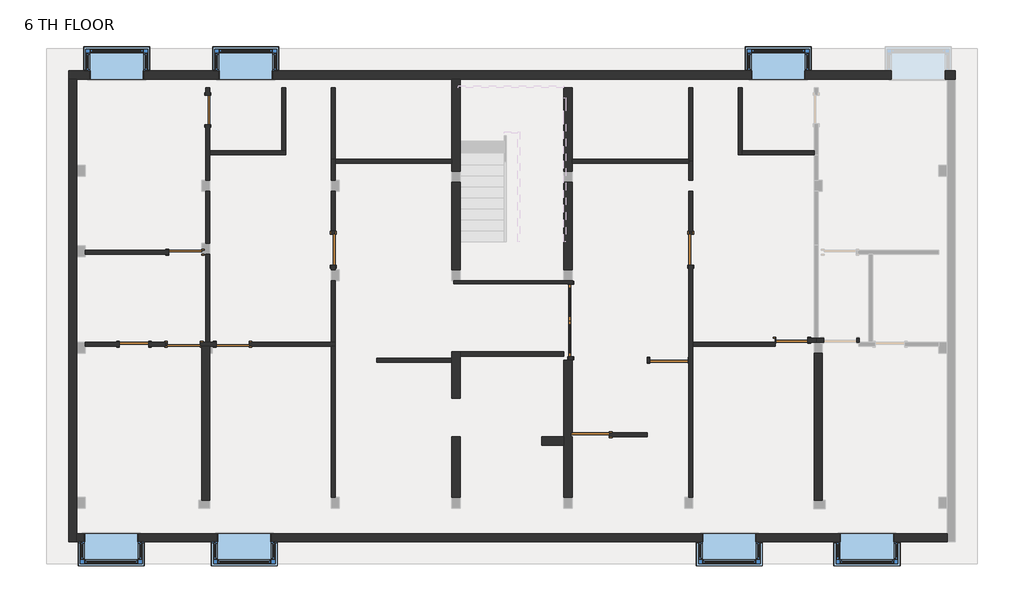
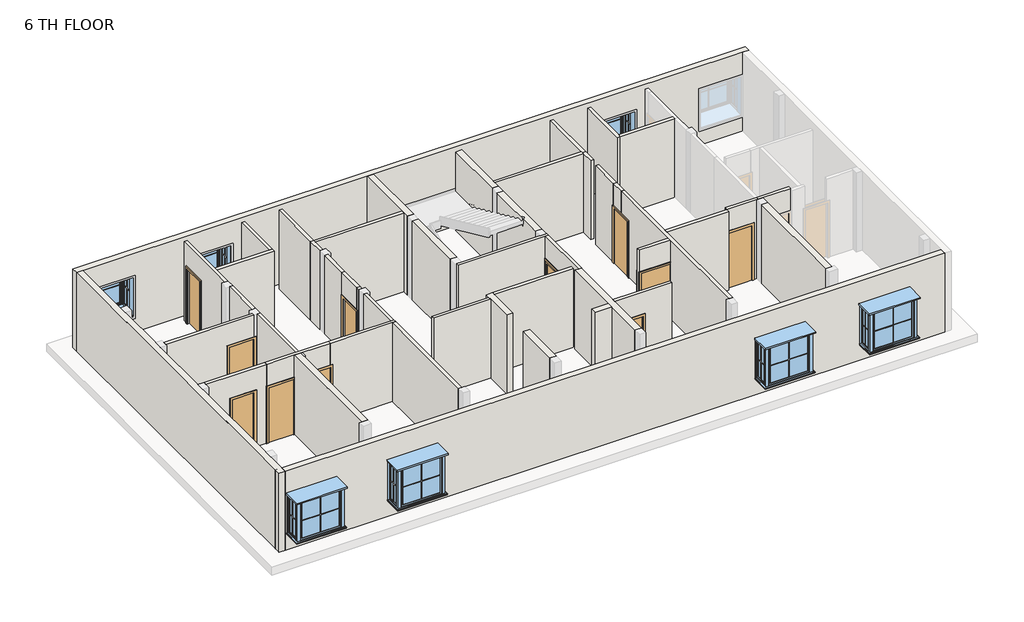
# One storey, part 1 of 2: 48 walls, 11 doors, 7 windows.
"""IFC4 building model written with IfcOpenShell, lengths in millimetres."""

from ifc_helpers import new_model, si_unit, frame, origin, place, context, project, spatial, polyline, outline, extrude, faceted_brep, transform, mapped, element, save
from components import door_04ab2522, m_door_single_panel_05506f71, door_07b5d71c, door_85b31ab1, door_1991e9a2, door_4c0a2014, door_82def9da, m_door_single_panel_3_x7_f8176753, m_door_single_panel_3_x7_ebb67e73, window_19bbd869

model = new_model("IFC4")

# Units and contexts
model_context = context("Model", 3, world=origin())
ifc_project = project(units=[si_unit("LENGTHUNIT", "METRE", prefix="MILLI")], contexts=[model_context])

# Site, building, storey
site = spatial("IfcSite", under=ifc_project)
building = spatial("IfcBuilding", under=site)
storey = spatial("IfcBuildingStorey", under=building, Name="6 TH FLOOR", Elevation=22402.8)

# Doors
placement = place(None, origin())
door_shape = door_04ab2522(model_context)
element("IfcDoor", 1, ObjectType="M_Door-Double-Glass : 6'7\"X7'", at=placement, inside=storey, context=model_context, shape_type="MappedRepresentation", body=[
    mapped(door_shape, transform((1217.5394962, 1183.3817656, 22402.8), x_axis=(0.0, 1.0, 0.0), y_axis=(-1.0, 0.0, 0.0), z_axis=(0.0, 0.0, 1.0))),
])
m_door_single_panel_shape = m_door_single_panel_05506f71(model_context)
element("IfcDoor", 2, ObjectType="M_Door-Single-Panel", at=placement, inside=storey, context=model_context, shape_type="MappedRepresentation", body=[
    mapped(m_door_single_panel_shape, transform((1745.3012085, -1975.7432663, 22402.8), x_axis=(-1.0, 0.0, 0.0), y_axis=(0.0, -1.0, 0.0), z_axis=(0.0, 0.0, 1.0))),
])
element("IfcDoor", 3, ObjectType="M_Door-Single-Panel", at=placement, inside=storey, context=model_context, shape_type="MappedRepresentation", body=[
    mapped(m_door_single_panel_shape, transform((3933.4813133, 90.9578621, 22402.8), x_axis=(1.0, 0.0, 0.0), y_axis=(0.0, 1.0, 0.0), z_axis=(0.0, 0.0, 1.0))),
])
door_2_shape = door_07b5d71c(model_context)
element("IfcDoor", 4, ObjectType="M_Door-Single-Panel : 2'10\"X7' 2", at=placement, inside=storey, context=model_context, shape_type="MappedRepresentation", body=[
    mapped(door_2_shape, transform((-5360.3487995, 3142.9626891, 22402.8), x_axis=(0.0, -1.0, 0.0), y_axis=(1.0, 0.0, 0.0), z_axis=(0.0, 0.0, 1.0))),
])
door_3_shape = door_85b31ab1(model_context)
element("IfcDoor", 5, ObjectType="M_Door-Single-Panel : 2'10\"X7' 2", at=placement, inside=storey, context=model_context, shape_type="MappedRepresentation", body=[
    mapped(door_3_shape, transform((4532.9512082, 3142.9626891, 22402.8), x_axis=(0.0, -1.0, 0.0), y_axis=(1.0, 0.0, 0.0), z_axis=(0.0, 0.0, 1.0))),
])
door_4_shape = door_1991e9a2(model_context)
element("IfcDoor", 6, ObjectType="M_Door-Single-Panel : 2'11\"X7' 3", at=placement, inside=storey, context=model_context, shape_type="MappedRepresentation", body=[
    mapped(door_4_shape, transform((7330.1405552, 640.4567334, 22402.8), x_axis=(1.0, 0.0, 0.0), y_axis=(0.0, 1.0, 0.0), z_axis=(0.0, 0.0, 1.0))),
])
door_5_shape = door_4c0a2014(model_context)
element("IfcDoor", 7, ObjectType="M_Door-Single-Panel : 2'8\"X7'", at=placement, inside=storey, context=model_context, shape_type="MappedRepresentation", body=[
    mapped(door_5_shape, transform((-10873.4462614, 526.1567334, 22402.8), x_axis=(1.0, 0.0, 0.0), y_axis=(0.0, 1.0, 0.0), z_axis=(0.0, 0.0, 1.0))),
])
door_6_shape = door_82def9da(model_context)
element("IfcDoor", 8, ObjectType="M_Door-Single-Panel : 2'8\"X7'", at=placement, inside=storey, context=model_context, shape_type="MappedRepresentation", body=[
    mapped(door_6_shape, transform((-8827.4487992, 7008.6751452, 22402.8), x_axis=(0.0, 1.0, 0.0), y_axis=(-1.0, 0.0, 0.0), z_axis=(0.0, 0.0, 1.0))),
])
m_door_single_panel_3_x7_shape = m_door_single_panel_3_x7_f8176753(model_context)
element("IfcDoor", 9, ObjectType="M_Door-Single-Panel : 3'X7'", at=placement, inside=storey, context=model_context, shape_type="MappedRepresentation", body=[
    mapped(m_door_single_panel_3_x7_shape, transform((-9456.0987989, 3078.8567332, 22402.8), x_axis=(1.0, 0.0, 0.0), y_axis=(0.0, 1.0, 0.0), z_axis=(0.0, 0.0, 1.0))),
])
element("IfcDoor", 10, ObjectType="M_Door-Single-Panel : 3'X7'", at=placement, inside=storey, context=model_context, shape_type="MappedRepresentation", body=[
    mapped(m_door_single_panel_3_x7_shape, transform((-8144.8381465, 526.1567334, 22402.8), x_axis=(-1.0, 0.0, 0.0), y_axis=(0.0, -1.0, 0.0), z_axis=(0.0, 0.0, 1.0))),
])
m_door_single_panel_3_x7_2_shape = m_door_single_panel_3_x7_ebb67e73(model_context)
element("IfcDoor", 11, ObjectType="M_Door-Single-Panel : 3'X7'", at=placement, inside=storey, context=model_context, shape_type="MappedRepresentation", body=[
    mapped(m_door_single_panel_3_x7_2_shape, transform((-9494.1987992, 526.1567334, 22402.8), x_axis=(1.0, 0.0, 0.0), y_axis=(0.0, 1.0, 0.0), z_axis=(0.0, 0.0, 1.0))),
])

# Walls
element("IfcWall", 12, ObjectType="3.5\"", at=placement, inside=storey, context=model_context, shape_type="Brep", body=[
    faceted_brep([(-2020.2487998, 2196.2067742, 22402.8), (1158.0082462, 2196.2067742, 22402.8), (1272.3082462, 2196.2067742, 22402.8), (1272.3082462, 2196.2067742, 25450.8), (1158.0082462, 2196.2067742, 25450.8), (-2020.2487998, 2196.2067742, 25450.8), (-2020.2487998, 2285.1067742, 22402.8), (-2020.2487998, 2285.1067742, 25450.8), (-1845.5417538, 2285.1067742, 25450.8), (1024.6582462, 2285.1067742, 25450.8), (1253.2582462, 2285.1067742, 25450.8), (1272.3082462, 2285.1067742, 25450.8), (1272.3082462, 2285.1067742, 22402.8), (1253.2582462, 2285.1067742, 22402.8), (1024.6582462, 2285.1067742, 22402.8), (-1845.5417538, 2285.1067742, 22402.8)], [[[0, 1, 2, 3, 4, 5]], [[6, 7, 8, 9, 10, 11, 12, 13, 14, 15]], [[2, 1, 0, 6, 15, 14, 13, 12]], [[5, 4, 3, 11, 10, 9, 8, 7]], [[0, 5, 7, 6]], [[3, 2, 12, 11]]]),
])
element("IfcWall", 13, ObjectType="4.5\"", at=placement, inside=storey, context=model_context, shape_type="SweptSolid", body=[
    extrude(outline(polyline([(3132.0737955, 25450.8), (3628.3344162, 25450.8), (3628.3344162, 22402.8), (3574.7626891, 22402.8), (3574.7626891, 24536.4), (3132.0737955, 24536.4), (3132.0737955, 25450.8)])), frame((4475.8012082, 0.0, 0.0), z_axis=(1.0, 0.0, 0.0), x_axis=(0.0, 1.0, 0.0)), (0.0, 0.0, 1.0), 114.3),
])
element("IfcWall", 14, ObjectType="4.5\"", at=placement, inside=storey, context=model_context, shape_type="SweptSolid", body=[
    extrude(outline(polyline([(2711.1626891, 25450.8), (3671.8272228, 25450.8), (3671.8272228, 22402.8), (3574.7626891, 22402.8), (3574.7626891, 24536.4), (2711.1626891, 24536.4), (2711.1626891, 25450.8)])), frame((-5417.4987995, 0.0, 0.0), z_axis=(1.0, 0.0, 0.0), x_axis=(0.0, 1.0, 0.0)), (0.0, 0.0, 1.0), 114.3),
])
element("IfcWall", 15, ObjectType="4.5\"", at=placement, inside=storey, context=model_context, shape_type="Brep", body=[
    faceted_brep([(-7690.1644155, 469.0067334, 25450.8), (-8713.148796, 469.0067334, 25450.8), (-8771.750543, 469.0067334, 25450.8), (-9000.350543, 469.0067334, 25450.8), (-10009.8462614, 469.0067334, 25450.8), (-10009.8462614, 469.0067334, 22402.8), (-9951.3987992, 469.0067334, 22402.8), (-9951.3987992, 469.0067334, 24536.4), (-9036.9987992, 469.0067334, 24536.4), (-9036.9987992, 469.0067334, 22402.8), (-9000.350543, 469.0067334, 22402.8), (-8771.750543, 469.0067334, 22402.8), (-8713.148796, 469.0067334, 22402.8), (-8602.0381465, 469.0067334, 22402.8), (-8602.0381465, 469.0067334, 24536.4), (-7690.1644155, 469.0067334, 24536.4), (-10009.8462614, 583.3067334, 25450.8), (-7690.1644155, 583.3067334, 25450.8), (-7690.1644155, 583.3067334, 24536.4), (-8602.0381465, 583.3067334, 24536.4), (-8602.0381465, 583.3067334, 22402.8), (-9036.9987992, 583.3067334, 22402.8), (-9036.9987992, 583.3067334, 24536.4), (-9951.3987992, 583.3067334, 24536.4), (-9951.3987992, 583.3067334, 22402.8), (-10009.8462614, 583.3067334, 22402.8)], [[[0, 1, 2, 3, 4, 5, 6, 7, 8, 9, 10, 11, 12, 13, 14, 15]], [[16, 17, 18, 19, 20, 21, 22, 23, 24, 25]], [[5, 25, 24, 6]], [[9, 21, 20, 13, 12, 11, 10]], [[17, 0, 15, 18]], [[4, 3, 2, 1, 0, 17, 16]], [[5, 4, 16, 25]], [[8, 22, 21, 9]], [[7, 23, 22, 8]], [[23, 7, 6, 24]], [[19, 14, 13, 20]], [[14, 19, 18, 15]]]),
])
element("IfcWall", 16, ObjectType="4.5\"", at=placement, inside=storey, context=model_context, shape_type="Brep", body=[
    faceted_brep([(8000.0512079, 583.3067334, 22402.8), (8000.0512079, 583.3067334, 25450.8), (7942.9012047, 583.3067334, 25450.8), (6862.7668241, 583.3067334, 25450.8), (6862.7668241, 583.3067334, 22402.8), (6885.6405552, 583.3067334, 22402.8), (6885.6405552, 583.3067334, 24536.4), (7774.6405552, 583.3067334, 24536.4), (7774.6405552, 583.3067334, 22402.8), (7942.9012047, 583.3067334, 22402.8), (8000.0512079, 697.6067334, 25450.8), (8000.0512079, 697.6067334, 22402.8), (7942.9012079, 697.6067334, 22402.8), (7774.6405552, 697.6067334, 22402.8), (7774.6405552, 697.6067334, 24536.4), (6885.6405552, 697.6067334, 24536.4), (6885.6405552, 697.6067334, 22402.8), (6862.7668241, 697.6067334, 22402.8), (6862.7668241, 697.6067334, 25450.8), (7942.9012079, 697.6067334, 25450.8)], [[[0, 1, 2, 3, 4, 5, 6, 7, 8, 9]], [[10, 11, 12, 13, 14, 15, 16, 17, 18, 19]], [[4, 17, 16, 5]], [[11, 0, 9, 8, 13, 12]], [[1, 0, 11, 10]], [[3, 2, 1, 10, 19, 18]], [[4, 3, 18, 17]], [[7, 14, 13, 8]], [[14, 7, 6, 15]], [[15, 6, 5, 16]]]),
])
element("IfcWall", 17, ObjectType="4.5\"", at=placement, inside=storey, context=model_context, shape_type="Brep", body=[
    faceted_brep([(9187.5012047, 583.3067334, 22402.8), (9187.5012047, 583.3067334, 25450.8), (8171.5012047, 583.3067334, 25450.8), (8000.0512079, 583.3067334, 25450.8), (8000.0512079, 583.3067334, 22402.8), (8171.5012047, 583.3067334, 22402.8), (8209.6012079, 583.3067334, 22402.8), (8209.6012079, 583.3067334, 24536.4), (9124.0012079, 583.3067334, 24536.4), (9124.0012079, 583.3067334, 22402.8), (9187.5012047, 697.6067334, 25450.8), (9187.5012047, 697.6067334, 22402.8), (9124.0012079, 697.6067334, 22402.8), (9124.0012079, 697.6067334, 24536.4), (8209.6012079, 697.6067334, 24536.4), (8209.6012079, 697.6067334, 22402.8), (8057.2012079, 697.6067334, 22402.8), (8000.0512079, 697.6067334, 22402.8), (8000.0512079, 697.6067334, 25450.8), (8057.2012079, 697.6067334, 25450.8)], [[[0, 1, 2, 3, 4, 5, 6, 7, 8, 9]], [[10, 11, 12, 13, 14, 15, 16, 17, 18, 19]], [[11, 0, 9, 12]], [[4, 17, 16, 15, 6, 5]], [[1, 0, 11, 10]], [[3, 2, 1, 10, 19, 18]], [[4, 3, 18, 17]], [[7, 14, 13, 8]], [[8, 13, 12, 9]], [[14, 7, 6, 15]]]),
])
element("IfcWall", 18, ObjectType="4.5\"", at=placement, inside=storey, context=model_context, shape_type="SweptSolid", body=[
    extrude(outline(polyline([(22402.8, 3334.0114184), (25450.8, 3334.0114184), (25450.8, 1250.0012085), (24536.4, 1250.0012085), (24536.4, 2278.7012085), (22402.8, 2278.7012085), (22402.8, 3334.0114184)])), frame((0.0, -2032.8932663, 0.0), z_axis=(0.0, 1.0, 0.0), x_axis=(0.0, 0.0, 1.0)), (0.0, 0.0, 1.0), 114.3),
])
element("IfcWall", 19, ObjectType="4.5\"", at=placement, inside=storey, context=model_context, shape_type="SweptSolid", body=[
    extrude(outline(polyline([(24536.4, 4466.8813133), (22402.8, 4466.8813133), (22402.8, 4475.8012082), (25450.8, 4475.8012082), (25450.8, 3334.0114184), (22402.8, 3334.0114184), (22402.8, 3400.0813133), (24536.4, 3400.0813133), (24536.4, 4466.8813133)])), frame((0.0, 33.8078621, 0.0), z_axis=(0.0, 1.0, 0.0), x_axis=(0.0, 0.0, 1.0)), (0.0, 0.0, 1.0), 114.3),
])
element("IfcWall", 20, ObjectType="4.5\"", at=placement, inside=storey, context=model_context, shape_type="SweptSolid", body=[
    extrude(outline(polyline([(1021.4012085, 202.3067742), (-1848.7987998, 202.3067742), (-1848.7987998, 316.6067742), (1021.4012085, 316.6067742), (1021.4012085, 202.3067742)])), frame((0.0, 0.0, 22402.8), z_axis=(0.0, 0.0, 1.0), x_axis=(1.0, 0.0, 0.0)), (0.0, 0.0, 1.0), 3048.0),
])
element("IfcWall", 21, ObjectType="4.5\"", at=placement, inside=storey, context=model_context, shape_type="Brep", body=[
    faceted_brep([(1158.0082462, 2196.2067742, 22402.8), (1158.0082462, 2186.6817656, 22402.8), (1158.0082462, 2186.6817656, 24536.4), (1158.0082462, 180.0817656, 24536.4), (1158.0082462, 180.0817656, 22402.8), (1158.0082462, 90.9578621, 22402.8), (1158.0082462, 90.9578621, 25450.8), (1158.0082462, 2196.2067742, 25450.8), (1272.3082462, 2186.6817656, 24536.4), (1272.3082462, 2186.6817656, 22402.8), (1272.3082462, 2196.2067742, 22402.8), (1272.3082462, 2196.2067742, 25450.8), (1272.3082462, 90.9578621, 25450.8), (1272.3082462, 90.9578621, 22402.8), (1272.3082462, 180.0817656, 22402.8), (1272.3082462, 180.0817656, 24536.4), (1250.0012085, 90.9578621, 22402.8), (1250.0012085, 90.9578621, 25450.8)], [[[0, 1, 2, 3, 4, 5, 6, 7]], [[8, 9, 10, 11, 12, 13, 14, 15]], [[14, 13, 16, 5, 4]], [[10, 9, 1, 0]], [[6, 5, 16, 13, 12, 17]], [[7, 6, 17, 12, 11]], [[0, 7, 11, 10]], [[2, 1, 9, 8]], [[3, 2, 8, 15]], [[4, 3, 15, 14]]]),
])
element("IfcWall", 22, ObjectType="4.5\"", at=placement, inside=storey, context=model_context, shape_type="Brep", body=[
    faceted_brep([(1250.0012085, 5536.3067329, 22402.8), (4475.8012082, 5536.3067329, 22402.8), (4475.8012082, 5536.3067329, 25450.8), (1250.0012085, 5536.3067329, 25450.8), (1250.0012085, 5650.6067329, 22402.8), (1250.0012085, 5650.6067329, 25450.8), (4475.8012082, 5650.6067329, 25450.8), (4475.8012082, 5650.6067329, 22402.8), (4475.8012082, 5593.4567329, 22402.8), (4475.8012082, 5593.4567329, 25450.8)], [[[0, 1, 2, 3]], [[4, 5, 6, 7]], [[1, 0, 4, 7, 8]], [[3, 2, 9, 6, 5]], [[2, 1, 8, 7, 6, 9]], [[0, 3, 5, 4]]]),
])
element("IfcWall", 23, ObjectType="4.5\"", at=placement, inside=storey, context=model_context, shape_type="SweptSolid", body=[
    extrude(outline(polyline([(-5417.4987995, -3709.2932193), (-5417.4987995, 469.0067334), (-5303.1987995, 469.0067334), (-5303.1987995, -3709.2932193), (-5417.4987995, -3709.2932193)])), frame((0.0, 0.0, 22402.8), z_axis=(0.0, 0.0, 1.0), x_axis=(1.0, 0.0, 0.0)), (0.0, 0.0, 1.0), 3048.0),
])
element("IfcWall", 24, ObjectType="4.5\" 2", at=placement, inside=storey, context=model_context, shape_type="SweptSolid", body=[
    extrude(outline(polyline([(25450.8, -8998.8987989), (25450.8, -12224.6987989), (22402.8, -12224.6987989), (22402.8, -9913.2987989), (24536.4, -9913.2987989), (24536.4, -8998.8987989), (25450.8, -8998.8987989)])), frame((0.0, 3021.7067332, 0.0), z_axis=(0.0, 1.0, 0.0), x_axis=(0.0, 0.0, 1.0)), (0.0, 0.0, 1.0), 114.3),
])
element("IfcWall", 25, ObjectType="4.5\" 2", at=placement, inside=storey, context=model_context, shape_type="SweptSolid", body=[
    extrude(outline(polyline([(-8770.2987992, 4761.606733), (-8770.2987992, 3326.5067332), (-8884.5987992, 3326.5067332), (-8884.5987992, 4761.606733), (-8770.2987992, 4761.606733)])), frame((0.0, 0.0, 22402.8), z_axis=(0.0, 0.0, 1.0), x_axis=(1.0, 0.0, 0.0)), (0.0, 0.0, 1.0), 3048.0),
])
element("IfcWall", 26, ObjectType="4.5\" 2", at=placement, inside=storey, context=model_context, shape_type="Brep", body=[
    faceted_brep([(-8770.2987992, 7415.0751452, 24536.4), (-8770.2987992, 7415.0751452, 22402.8), (-8770.2987992, 7631.8067329, 22402.8), (-8770.2987992, 7631.8067329, 25450.8), (-8770.2987992, 5879.2067329, 25450.8), (-8770.2987992, 5764.9067329, 25450.8), (-8770.2987992, 5066.406733, 25450.8), (-8770.2987992, 5066.406733, 22402.8), (-8770.2987992, 5764.9067329, 22402.8), (-8770.2987992, 5879.2067329, 22402.8), (-8770.2987992, 6602.2751452, 22402.8), (-8770.2987992, 6602.2751452, 24536.4), (-8884.5987992, 7631.8067329, 22402.8), (-8884.5987992, 7415.0751452, 22402.8), (-8884.5987992, 7415.0751452, 24536.4), (-8884.5987992, 6602.2751452, 24536.4), (-8884.5987992, 6602.2751452, 22402.8), (-8884.5987992, 5066.406733, 22402.8), (-8884.5987992, 5066.406733, 25450.8), (-8884.5987992, 7631.8067329, 25450.8)], [[[0, 1, 2, 3, 4, 5, 6, 7, 8, 9, 10, 11]], [[12, 13, 14, 15, 16, 17, 18, 19]], [[2, 1, 13, 12]], [[10, 9, 8, 7, 17, 16]], [[3, 2, 12, 19]], [[6, 5, 4, 3, 19, 18]], [[7, 6, 18, 17]], [[14, 13, 1, 0]], [[15, 14, 0, 11]], [[16, 15, 11, 10]]]),
])
element("IfcWall", 27, ObjectType="4.5\" 2", at=placement, inside=storey, context=model_context, shape_type="Brep", body=[
    faceted_brep([(-8770.2987992, 5764.9067329, 22402.8), (-6674.7987994, 5764.9067329, 22402.8), (-6674.7987994, 5764.9067329, 25450.8), (-8770.2987992, 5764.9067329, 25450.8), (-8770.2987992, 5879.2067329, 22402.8), (-8770.2987992, 5879.2067329, 25450.8), (-6789.0987994, 5879.2067329, 25450.8), (-6674.7987994, 5879.2067329, 25450.8), (-6674.7987994, 5879.2067329, 22402.8), (-6789.0987994, 5879.2067329, 22402.8)], [[[0, 1, 2, 3]], [[4, 5, 6, 7, 8, 9]], [[1, 0, 4, 9, 8]], [[3, 2, 7, 6, 5]], [[0, 3, 5, 4]], [[2, 1, 8, 7]]]),
])
element("IfcWall", 28, ObjectType="4.5\" 2", at=placement, inside=storey, context=model_context, shape_type="SweptSolid", body=[
    extrude(outline(polyline([(-6674.7987994, 7631.8067329), (-6674.7987994, 5879.2067329), (-6789.0987994, 5879.2067329), (-6789.0987994, 7631.8067329), (-6674.7987994, 7631.8067329)])), frame((0.0, 0.0, 22402.8), z_axis=(0.0, 0.0, 1.0), x_axis=(1.0, 0.0, 0.0)), (0.0, 0.0, 1.0), 3048.0),
])
element("IfcWall", 29, ObjectType="4.5\" 2", at=placement, inside=storey, context=model_context, shape_type="SweptSolid", body=[
    extrude(outline(polyline([(24536.4, -10467.0462614), (22402.8, -10467.0462614), (22402.8, -10009.8462614), (25450.8, -10009.8462614), (25450.8, -12224.6987989), (22402.8, -12224.6987989), (22402.8, -11279.8462614), (24536.4, -11279.8462614), (24536.4, -10467.0462614)])), frame((0.0, 469.0067334, 0.0), z_axis=(0.0, 1.0, 0.0), x_axis=(0.0, 0.0, 1.0)), (0.0, 0.0, 1.0), 114.3),
])
element("IfcWall", 30, ObjectType="4.5\" 2", at=placement, inside=storey, context=model_context, shape_type="SweptSolid", body=[
    extrude(outline(polyline([(-8770.298796, 3021.7067332), (-8770.298796, 583.3067804), (-8884.598796, 583.3067804), (-8884.598796, 3021.7067332), (-8770.298796, 3021.7067332)])), frame((0.0, 0.0, 22402.8), z_axis=(0.0, 0.0, 1.0), x_axis=(1.0, 0.0, 0.0)), (0.0, 0.0, 1.0), 3048.0),
])
element("IfcWall", 31, ObjectType="4.5\" 2", at=placement, inside=storey, context=model_context, shape_type="Brep", body=[
    faceted_brep([(-5303.1987995, 469.0067334, 25450.8), (-5417.4987995, 469.0067334, 25450.8), (-7690.1644155, 469.0067334, 25450.8), (-7690.1644155, 469.0067334, 24536.4), (-7687.6381465, 469.0067334, 24536.4), (-7687.6381465, 469.0067334, 22402.8), (-5417.4987995, 469.0067334, 22402.8), (-5303.1987995, 469.0067334, 22402.8), (-7690.1644155, 583.3067334, 25450.8), (-5417.4987995, 583.3067334, 25450.8), (-5303.1987995, 583.3067334, 25450.8), (-5303.1987995, 583.3067334, 22402.8), (-5417.4987995, 583.3067334, 22402.8), (-7687.6381465, 583.3067334, 22402.8), (-7687.6381465, 583.3067334, 24536.4), (-7690.1644155, 583.3067334, 24536.4)], [[[0, 1, 2, 3, 4, 5, 6, 7]], [[8, 9, 10, 11, 12, 13, 14, 15]], [[11, 7, 6, 5, 13, 12]], [[2, 1, 0, 10, 9, 8]], [[2, 8, 15, 3]], [[0, 7, 11, 10]], [[14, 4, 3, 15]], [[4, 14, 13, 5]]]),
])
element("IfcWall", 32, ObjectType="4.5\" 2", at=placement, inside=storey, context=model_context, shape_type="SweptSolid", body=[
    extrude(outline(polyline([(-5303.1987995, 2285.1067802), (-5303.1987995, 583.3067334), (-5417.4987995, 583.3067334), (-5417.4987995, 2285.1067802), (-5303.1987995, 2285.1067802)])), frame((0.0, 0.0, 22402.8), z_axis=(0.0, 0.0, 1.0), x_axis=(1.0, 0.0, 0.0)), (0.0, 0.0, 1.0), 3048.0),
])
element("IfcWall", 33, ObjectType="4.5\" 2", at=placement, inside=storey, context=model_context, shape_type="Brep", body=[
    faceted_brep([(-5303.1987995, 2589.9067802, 22402.8), (-5303.1987995, 2711.1626891, 22402.8), (-5303.1987995, 2711.1626891, 24536.4), (-5303.1987995, 2711.1626891, 25450.8), (-5303.1987995, 2589.9067802, 25450.8), (-5417.4987995, 2589.9067802, 22402.8), (-5417.4987995, 2589.9067802, 25450.8), (-5417.4987995, 2711.1626891, 25450.8), (-5417.4987995, 2711.1626891, 24536.4), (-5417.4987995, 2711.1626891, 22402.8)], [[[0, 1, 2, 3, 4]], [[5, 6, 7, 8, 9]], [[1, 0, 5, 9]], [[3, 2, 1, 9, 8, 7]], [[4, 3, 7, 6]], [[0, 4, 6, 5]]]),
])
element("IfcWall", 34, ObjectType="4.5\" 2", at=placement, inside=storey, context=model_context, shape_type="SweptSolid", body=[
    extrude(outline(polyline([(-5303.1987995, 4761.606733), (-5303.1987995, 3671.8272228), (-5417.4987995, 3671.8272228), (-5417.4987995, 4761.606733), (-5303.1987995, 4761.606733)])), frame((0.0, 0.0, 22402.8), z_axis=(0.0, 0.0, 1.0), x_axis=(1.0, 0.0, 0.0)), (0.0, 0.0, 1.0), 3048.0),
])
element("IfcWall", 35, ObjectType="4.5\" 2", at=placement, inside=storey, context=model_context, shape_type="Brep", body=[
    faceted_brep([(-5303.1987995, 5066.406733, 22402.8), (-5303.1987995, 5536.3067329, 22402.8), (-5303.1987995, 5650.6067329, 22402.8), (-5303.1987995, 5650.6067329, 25450.8), (-5303.1987995, 5536.3067329, 25450.8), (-5303.1987995, 5066.406733, 25450.8), (-5417.4987995, 5066.406733, 22402.8), (-5417.4987995, 5066.406733, 25450.8), (-5417.4987995, 5650.6067329, 25450.8), (-5417.4987995, 5650.6067329, 22402.8)], [[[0, 1, 2, 3, 4, 5]], [[6, 7, 8, 9]], [[2, 1, 0, 6, 9]], [[5, 4, 3, 8, 7]], [[0, 5, 7, 6]], [[3, 2, 9, 8]]]),
])
element("IfcWall", 36, ObjectType="4.5\" 2", at=placement, inside=storey, context=model_context, shape_type="SweptSolid", body=[
    extrude(outline(polyline([(-2077.3987998, 5536.3067329), (-5303.1987995, 5536.3067329), (-5303.1987995, 5650.6067329), (-2077.3987998, 5650.6067329), (-2077.3987998, 5536.3067329)])), frame((0.0, 0.0, 22402.8), z_axis=(0.0, 0.0, 1.0), x_axis=(1.0, 0.0, 0.0)), (0.0, 0.0, 1.0), 3048.0),
])
element("IfcWall", 37, ObjectType="4.5\" 2", at=placement, inside=storey, context=model_context, shape_type="SweptSolid", body=[
    extrude(outline(polyline([(-5417.4987995, 5650.6067329), (-5417.4987995, 7631.8067329), (-5303.1987995, 7631.8067329), (-5303.1987995, 5650.6067329), (-5417.4987995, 5650.6067329)])), frame((0.0, 0.0, 22402.8), z_axis=(0.0, 0.0, 1.0), x_axis=(1.0, 0.0, 0.0)), (0.0, 0.0, 1.0), 3048.0),
])
element("IfcWall", 38, ObjectType="4.5\" 2", at=placement, inside=storey, context=model_context, shape_type="Brep", body=[
    faceted_brep([(4475.8012082, 5593.4567329, 22402.8), (4475.8012082, 5536.3067329, 22402.8), (4475.8012082, 5066.40678, 22402.8), (4475.8012082, 5066.40678, 25450.8), (4475.8012082, 5536.3067329, 25450.8), (4475.8012082, 5593.4567329, 25450.8), (4590.1012082, 5593.4567329, 22402.8), (4590.1012082, 5593.4567329, 25450.8), (4590.1012082, 5066.40678, 25450.8), (4590.1012082, 5066.40678, 22402.8)], [[[0, 1, 2, 3, 4, 5]], [[6, 7, 8, 9]], [[2, 1, 0, 6, 9]], [[3, 2, 9, 8]], [[5, 4, 3, 8, 7]], [[0, 5, 7, 6]]]),
])
element("IfcWall", 39, ObjectType="4.5\" 2", at=placement, inside=storey, context=model_context, shape_type="SweptSolid", body=[
    extrude(outline(polyline([(4475.8012082, 3628.3344162), (4475.8012082, 4761.606733), (4590.1012082, 4761.606733), (4590.1012082, 3628.3344162), (4475.8012082, 3628.3344162)])), frame((0.0, 0.0, 22402.8), z_axis=(0.0, 0.0, 1.0), x_axis=(1.0, 0.0, 0.0)), (0.0, 0.0, 1.0), 3048.0),
])
element("IfcWall", 40, ObjectType="4.5\" 2", at=placement, inside=storey, context=model_context, shape_type="Brep", body=[
    faceted_brep([(4475.8012082, -3709.2932193, 22402.8), (4475.8012082, -3709.2932193, 25450.8), (4475.8012082, 33.8078621, 25450.8), (4475.8012082, 148.1078621, 25450.8), (4475.8012082, 3132.0737955, 25450.8), (4475.8012082, 3132.0737955, 24536.4), (4475.8012082, 2711.1626891, 24536.4), (4475.8012082, 2711.1626891, 22402.8), (4475.8012082, 148.1078621, 22402.8), (4475.8012082, 33.8078621, 22402.8), (4590.1012082, -3709.2932193, 25450.8), (4590.1012082, -3709.2932193, 22402.8), (4590.1012082, 469.0067334, 22402.8), (4590.1012082, 583.3067334, 22402.8), (4590.1012082, 2711.1626891, 22402.8), (4590.1012082, 2711.1626891, 24536.4), (4590.1012082, 3132.0737955, 24536.4), (4590.1012082, 3132.0737955, 25450.8), (4590.1012082, 583.3067334, 25450.8), (4590.1012082, 469.0067334, 25450.8)], [[[0, 1, 2, 3, 4, 5, 6, 7, 8, 9]], [[10, 11, 12, 13, 14, 15, 16, 17, 18, 19]], [[11, 0, 9, 8, 7, 14, 13, 12]], [[1, 0, 11, 10]], [[4, 3, 2, 1, 10, 19, 18, 17]], [[4, 17, 16, 5]], [[6, 15, 14, 7]], [[15, 6, 5, 16]]]),
])
element("IfcWall", 41, ObjectType="4.5\" 2", at=placement, inside=storey, context=model_context, shape_type="SweptSolid", body=[
    extrude(outline(polyline([(6862.7668241, 469.0067334), (4590.1012082, 469.0067334), (4590.1012082, 583.3067334), (6862.7668241, 583.3067334), (6862.7668241, 469.0067334)])), frame((0.0, 0.0, 22402.8), z_axis=(0.0, 0.0, 1.0), x_axis=(1.0, 0.0, 0.0)), (0.0, 0.0, 1.0), 3048.0),
])
element("IfcWall", 42, ObjectType="4.5\" 2", at=placement, inside=storey, context=model_context, shape_type="Brep", body=[
    faceted_brep([(4590.1012082, 5593.4567329, 22402.8), (4590.1012082, 7631.8067329, 22402.8), (4590.1012082, 7631.8067329, 25450.8), (4590.1012082, 5593.4567329, 25450.8), (4475.8012082, 5593.4567329, 22402.8), (4475.8012082, 5593.4567329, 25450.8), (4475.8012082, 5650.6067329, 25450.8), (4475.8012082, 7631.8067329, 25450.8), (4475.8012082, 7631.8067329, 22402.8), (4475.8012082, 5650.6067329, 22402.8)], [[[0, 1, 2, 3]], [[4, 5, 6, 7, 8, 9]], [[1, 0, 4, 9, 8]], [[2, 1, 8, 7]], [[3, 2, 7, 6, 5]], [[0, 3, 5, 4]]]),
])
element("IfcWall", 43, ObjectType="4.5\" 2", at=placement, inside=storey, context=model_context, shape_type="Brep", body=[
    faceted_brep([(5847.401208, 7631.8067329, 22402.8), (5847.401208, 5764.9067329, 22402.8), (5847.401208, 5764.9067329, 25450.8), (5847.401208, 7631.8067329, 25450.8), (5961.701208, 7631.8067329, 22402.8), (5961.701208, 7631.8067329, 25450.8), (5961.701208, 5879.2067329, 25450.8), (5961.701208, 5764.9067329, 25450.8), (5961.701208, 5764.9067329, 22402.8), (5961.701208, 5879.2067329, 22402.8)], [[[0, 1, 2, 3]], [[4, 5, 6, 7, 8, 9]], [[1, 0, 4, 9, 8]], [[3, 2, 7, 6, 5]], [[0, 3, 5, 4]], [[2, 1, 8, 7]]]),
])
element("IfcWall", 44, ObjectType="4.5\" 2", at=placement, inside=storey, context=model_context, shape_type="SweptSolid", body=[
    extrude(outline(polyline([(7942.9012079, 5764.9067329), (5961.701208, 5764.9067329), (5961.701208, 5879.2067329), (7942.9012079, 5879.2067329), (7942.9012079, 5764.9067329)])), frame((0.0, 0.0, 22402.8), z_axis=(0.0, 0.0, 1.0), x_axis=(1.0, 0.0, 0.0)), (0.0, 0.0, 1.0), 3048.0),
])
element("IfcWall", 45, ObjectType="4.5\" 2", at=placement, inside=storey, context=model_context, shape_type="SweptSolid", body=[
    extrude(outline(polyline([(-2077.3987998, 33.8078621), (-4161.4090098, 33.8078621), (-4161.4090098, 148.1078621), (-2077.3987998, 148.1078621), (-2077.3987998, 33.8078621)])), frame((0.0, 0.0, 22402.8), z_axis=(0.0, 0.0, 1.0), x_axis=(1.0, 0.0, 0.0)), (0.0, 0.0, 1.0), 3048.0),
])
element("IfcWall", 46, ObjectType="9\"", at=placement, inside=storey, context=model_context, shape_type="Brep", body=[
    faceted_brep([(-12681.8987957, 7860.4067329, 22402.8), (-12453.2987957, 7860.4067329, 22402.8), (-2074.1417538, 7860.4067329, 22402.8), (-1845.5417538, 7860.4067329, 22402.8), (11625.9012075, 7860.4067329, 22402.8), (11854.5012075, 7860.4067329, 22402.8), (11854.5012075, 7860.4067329, 25450.8), (11625.9012075, 7860.4067329, 25450.8), (-1845.5417538, 7860.4067329, 25450.8), (-2074.1417538, 7860.4067329, 25450.8), (-12453.2987957, 7860.4067329, 25450.8), (-12681.8987957, 7860.4067329, 25450.8), (11575.8012075, 7860.4067329, 24553.6), (11575.8012075, 7860.4067329, 23002.8), (10075.8012075, 7860.4067329, 23002.8), (10075.8012075, 7860.4067329, 24553.6), (7702.301208, 7860.4067329, 24553.6), (7702.301208, 7860.4067329, 23002.8), (6202.301208, 7860.4067329, 23002.8), (6202.301208, 7860.4067329, 24553.6), (-7029.6987993, 7860.4067329, 24553.6), (-7029.6987993, 7860.4067329, 23002.8), (-8529.6987993, 7860.4067329, 23002.8), (-8529.6987993, 7860.4067329, 24553.6), (-10598.3987957, 7860.4067329, 24553.6), (-10598.3987957, 7860.4067329, 23002.8), (-12098.3987957, 7860.4067329, 23002.8), (-12098.3987957, 7860.4067329, 24553.6), (-12681.8987957, 8089.0067329, 22402.8), (-12681.8987957, 8089.0067329, 25450.8), (11854.5012075, 8089.0067329, 25450.8), (11854.5012075, 8089.0067329, 22402.8), (11575.8012075, 8089.0067329, 24553.6), (10075.8012075, 8089.0067329, 24553.6), (10075.8012075, 8089.0067329, 23002.8), (11575.8012075, 8089.0067329, 23002.8), (7702.301208, 8089.0067329, 24553.6), (6202.301208, 8089.0067329, 24553.6), (6202.301208, 8089.0067329, 23002.8), (7702.301208, 8089.0067329, 23002.8), (-7029.6987993, 8089.0067329, 24553.6), (-8529.6987993, 8089.0067329, 24553.6), (-8529.6987993, 8089.0067329, 23002.8), (-7029.6987993, 8089.0067329, 23002.8), (-10598.3987957, 8089.0067329, 24553.6), (-12098.3987957, 8089.0067329, 24553.6), (-12098.3987957, 8089.0067329, 23002.8), (-10598.3987957, 8089.0067329, 23002.8)], [[[0, 1, 2, 3, 4, 5, 6, 7, 8, 9, 10, 11], [12, 13, 14, 15], [16, 17, 18, 19], [20, 21, 22, 23], [24, 25, 26, 27]], [[28, 29, 30, 31], [32, 33, 34, 35], [36, 37, 38, 39], [40, 41, 42, 43], [44, 45, 46, 47]], [[5, 4, 3, 2, 1, 0, 28, 31]], [[11, 10, 9, 8, 7, 6, 30, 29]], [[6, 5, 31, 30]], [[0, 11, 29, 28]], [[13, 12, 32, 35]], [[14, 13, 35, 34]], [[15, 14, 34, 33]], [[12, 15, 33, 32]], [[17, 16, 36, 39]], [[18, 17, 39, 38]], [[19, 18, 38, 37]], [[16, 19, 37, 36]], [[21, 20, 40, 43]], [[22, 21, 43, 42]], [[23, 22, 42, 41]], [[20, 23, 41, 40]], [[25, 24, 44, 47]], [[26, 25, 47, 46]], [[27, 26, 46, 45]], [[24, 27, 45, 44]]]),
])
element("IfcWall", 47, ObjectType="9\"", at=placement, inside=storey, context=model_context, shape_type="Brep", body=[
    faceted_brep([(-12453.2987957, -4941.1932661, 22402.8), (-12453.2987957, -4712.5932661, 22402.8), (-12453.2987957, -4014.0932671, 22402.8), (-12453.2987957, -3709.2932671, 22402.8), (-12453.2987957, 278.5067334, 22402.8), (-12453.2987957, 583.3067334, 22402.8), (-12453.2987957, 2951.8567332, 22402.8), (-12453.2987957, 3256.6567332, 22402.8), (-12453.2987957, 5174.3567339, 22402.8), (-12453.2987957, 5479.1567339, 22402.8), (-12453.2987957, 7860.4067329, 22402.8), (-12453.2987957, 7860.4067329, 25450.8), (-12453.2987957, 5479.1567339, 25450.8), (-12453.2987957, 5174.3567339, 25450.8), (-12453.2987957, 3256.6567332, 25450.8), (-12453.2987957, 2951.8567332, 25450.8), (-12453.2987957, 583.3067334, 25450.8), (-12453.2987957, 278.5067334, 25450.8), (-12453.2987957, -3709.2932671, 25450.8), (-12453.2987957, -4014.0932671, 25450.8), (-12453.2987957, -4712.5932661, 25450.8), (-12453.2987957, -4941.1932661, 25450.8), (-12681.8987957, -4941.1932661, 22402.8), (-12681.8987957, -4941.1932661, 25450.8), (-12681.8987957, 7860.4067329, 25450.8), (-12681.8987957, 7860.4067329, 22402.8)], [[[0, 1, 2, 3, 4, 5, 6, 7, 8, 9, 10, 11, 12, 13, 14, 15, 16, 17, 18, 19, 20, 21]], [[22, 23, 24, 25]], [[10, 9, 8, 7, 6, 5, 4, 3, 2, 1, 0, 22, 25]], [[21, 20, 19, 18, 17, 16, 15, 14, 13, 12, 11, 24, 23]], [[11, 10, 25, 24]], [[0, 21, 23, 22]]]),
])
element("IfcWall", 48, ObjectType="9\"", at=placement, inside=storey, context=model_context, shape_type="Brep", body=[
    faceted_brep([(-12453.2987957, -4712.5932661, 22402.8), (-12453.2987957, -4014.0932671, 22402.8), (-12453.2987957, -3709.2932671, 22402.8), (-12453.2987957, 278.5067334, 22402.8), (-12453.2987957, 583.3067334, 22402.8), (-12453.2987957, 2951.8567332, 22402.8), (-12453.2987957, 3256.6567332, 22402.8), (-12453.2987957, 5174.3567339, 22402.8), (-12453.2987957, 5479.1567339, 22402.8), (-12453.2987957, 7860.4067329, 22402.8), (-12453.2987957, 7860.4067329, 25450.8), (-12453.2987957, 5479.1567339, 25450.8), (-12453.2987957, 5174.3567339, 25450.8), (-12453.2987957, 3256.6567332, 25450.8), (-12453.2987957, 2951.8567332, 25450.8), (-12453.2987957, 583.3067334, 25450.8), (-12453.2987957, 278.5067334, 25450.8), (-12453.2987957, -3709.2932671, 25450.8), (-12453.2987957, -4014.0932671, 25450.8), (-12453.2987957, -4712.5932661, 25450.8), (-12681.8987957, -4712.5932661, 22402.8), (-12681.8987957, -4712.5932661, 25450.8), (-12681.8987957, 7860.4067329, 25450.8), (-12681.8987957, 7860.4067329, 22402.8)], [[[0, 1, 2, 3, 4, 5, 6, 7, 8, 9, 10, 11, 12, 13, 14, 15, 16, 17, 18, 19]], [[20, 21, 22, 23]], [[9, 8, 7, 6, 5, 4, 3, 2, 1, 0, 20, 23]], [[19, 18, 17, 16, 15, 14, 13, 12, 11, 10, 22, 21]], [[10, 9, 23, 22]], [[0, 19, 21, 20]]]),
])
element("IfcWall", 49, ObjectType="9\"", at=placement, inside=storey, context=model_context, shape_type="Brep", body=[
    faceted_brep([(-9000.350543, 469.0067334, 22402.8), (-9000.350543, -3785.4932196, 22402.8), (-9000.350543, -3785.4932196, 25450.8), (-9000.350543, 469.0067334, 25450.8), (-8771.750543, 469.0067334, 22402.8), (-8771.750543, 469.0067334, 25450.8), (-8771.750543, 278.5067334, 25450.8), (-8771.750543, -3785.4932196, 25450.8), (-8771.750543, -3785.4932196, 22402.8), (-8771.750543, 278.5067334, 22402.8)], [[[0, 1, 2, 3]], [[4, 5, 6, 7, 8, 9]], [[1, 0, 4, 9, 8]], [[2, 1, 8, 7]], [[3, 2, 7, 6, 5]], [[0, 3, 5, 4]]]),
])
element("IfcWall", 50, ObjectType="9\"", at=placement, inside=storey, context=model_context, shape_type="Brep", body=[
    faceted_brep([(-2077.3987998, 316.6067742, 22402.8), (-2077.3987998, 148.1078621, 22402.8), (-2077.3987998, 33.8078621, 22402.8), (-2077.3987998, -972.2341552, 22402.8), (-2077.3987998, -972.2341552, 25450.8), (-2077.3987998, 33.8078621, 25450.8), (-2077.3987998, 148.1078621, 25450.8), (-2077.3987998, 316.6067742, 25450.8), (-1848.7987998, 316.6067742, 22402.8), (-1848.7987998, 316.6067742, 25450.8), (-1848.7987998, 202.3067742, 25450.8), (-1848.7987998, -972.2341552, 25450.8), (-1848.7987998, -972.2341552, 22402.8), (-1848.7987998, 202.3067742, 22402.8)], [[[0, 1, 2, 3, 4, 5, 6, 7]], [[8, 9, 10, 11, 12, 13]], [[3, 2, 1, 0, 8, 13, 12]], [[4, 3, 12, 11]], [[7, 6, 5, 4, 11, 10, 9]], [[0, 7, 9, 8]]]),
])
element("IfcWall", 51, ObjectType="9\"", at=placement, inside=storey, context=model_context, shape_type="SweptSolid", body=[
    extrude(outline(polyline([(-2077.3987998, -3709.2932663), (-2077.3987998, -2032.8932663), (-1848.7987998, -2032.8932663), (-1848.7987998, -3709.2932663), (-2077.3987998, -3709.2932663)])), frame((0.0, 0.0, 22402.8), z_axis=(0.0, 0.0, 1.0), x_axis=(1.0, 0.0, 0.0)), (0.0, 0.0, 1.0), 3048.0),
])
element("IfcWall", 52, ObjectType="9\"", at=placement, inside=storey, context=model_context, shape_type="SweptSolid", body=[
    extrude(outline(polyline([(1021.4012085, -2261.4932663), (412.152227, -2261.4932663), (412.152227, -2032.8932663), (1021.4012085, -2032.8932663), (1021.4012085, -2261.4932663)])), frame((0.0, 0.0, 22402.8), z_axis=(0.0, 0.0, 1.0), x_axis=(1.0, 0.0, 0.0)), (0.0, 0.0, 1.0), 3048.0),
])
element("IfcWall", 53, ObjectType="9\"", at=placement, inside=storey, context=model_context, shape_type="Brep", body=[
    faceted_brep([(1021.4012085, 90.9578621, 22402.8), (1021.4012085, -2032.8932663, 22402.8), (1021.4012085, -2261.4932663, 22402.8), (1021.4012085, -3709.2932193, 22402.8), (1021.4012085, -3709.2932193, 25450.8), (1021.4012085, -2261.4932663, 25450.8), (1021.4012085, -2032.8932663, 25450.8), (1021.4012085, 90.9578621, 25450.8), (1250.0012085, -3709.2932193, 25450.8), (1250.0012085, -3709.2932193, 22402.8), (1250.0012085, -2032.8932663, 22402.8), (1250.0012085, -2032.8932663, 24536.4), (1250.0012085, -1918.5932663, 24536.4), (1250.0012085, -1918.5932663, 22402.8), (1250.0012085, 90.9578621, 22402.8), (1250.0012085, 90.9578621, 25450.8), (1250.0012085, -1918.5932663, 25450.8), (1250.0012085, -2032.8932663, 25450.8), (1158.0082462, 90.9578621, 22402.8), (1211.9012085, -1918.5932663, 22402.8), (1211.9012085, -2032.8932663, 22402.8), (1158.0082462, 90.9578621, 25450.8), (1211.9012085, -1918.5932663, 24536.4), (1211.9012085, -2032.8932663, 24536.4)], [[[0, 1, 2, 3, 4, 5, 6, 7]], [[8, 9, 10, 11, 12, 13, 14, 15, 16, 17]], [[3, 2, 1, 0, 18, 14, 13, 19, 20, 10, 9]], [[4, 3, 9, 8]], [[7, 6, 5, 4, 8, 17, 16, 15, 21]], [[0, 7, 21, 15, 14, 18]], [[22, 19, 13, 12]], [[20, 23, 11, 10]], [[19, 22, 23, 20]], [[23, 22, 12, 11]]]),
])
element("IfcWall", 54, ObjectType="9\"", at=placement, inside=storey, context=model_context, shape_type="SweptSolid", body=[
    extrude(outline(polyline([(-2074.1417538, 5320.4067329), (-2074.1417538, 7860.4067329), (-1845.5417538, 7860.4067329), (-1845.5417538, 5320.4067329), (-2074.1417538, 5320.4067329)])), frame((0.0, 0.0, 22402.8), z_axis=(0.0, 0.0, 1.0), x_axis=(1.0, 0.0, 0.0)), (0.0, 0.0, 1.0), 3048.0),
])
element("IfcWall", 55, ObjectType="9\"", at=placement, inside=storey, context=model_context, shape_type="SweptSolid", body=[
    extrude(outline(polyline([(-2074.1417538, 2589.906774), (-2074.1417538, 5015.606774), (-1845.5417538, 5015.606774), (-1845.5417538, 2589.906774), (-2074.1417538, 2589.906774)])), frame((0.0, 0.0, 22402.8), z_axis=(0.0, 0.0, 1.0), x_axis=(1.0, 0.0, 0.0)), (0.0, 0.0, 1.0), 3048.0),
])
element("IfcWall", 56, ObjectType="9\"", at=placement, inside=storey, context=model_context, shape_type="Brep", body=[
    faceted_brep([(1021.4012085, 7631.8067329, 22402.8), (1021.4012085, 5320.4067329, 22402.8), (1021.4012085, 5320.4067329, 25450.8), (1021.4012085, 7631.8067329, 25450.8), (1250.0012085, 7631.8067329, 22402.8), (1250.0012085, 7631.8067329, 25450.8), (1250.0012085, 5650.6067329, 25450.8), (1250.0012085, 5536.3067329, 25450.8), (1250.0012085, 5320.4067329, 25450.8), (1250.0012085, 5320.4067329, 22402.8), (1250.0012085, 5536.3067329, 22402.8), (1250.0012085, 5650.6067329, 22402.8)], [[[0, 1, 2, 3]], [[4, 5, 6, 7, 8, 9, 10, 11]], [[1, 0, 4, 11, 10, 9]], [[2, 1, 9, 8]], [[3, 2, 8, 7, 6, 5]], [[0, 3, 5, 4]]]),
])
element("IfcWall", 57, ObjectType="9\"", at=placement, inside=storey, context=model_context, shape_type="Brep", body=[
    faceted_brep([(1021.4012085, 5015.6067329, 22402.8), (1021.4012085, 2589.9067742, 22402.8), (1021.4012085, 2589.9067742, 25450.8), (1021.4012085, 5015.6067329, 25450.8), (1250.0012085, 5015.6067329, 22402.8), (1250.0012085, 5015.6067329, 25450.8), (1250.0012085, 2589.9067742, 25450.8), (1250.0012085, 2589.9067742, 22402.8), (1024.6582462, 2589.9067742, 22402.8), (1024.6582462, 2589.9067742, 25450.8)], [[[0, 1, 2, 3]], [[4, 5, 6, 7]], [[1, 0, 4, 7, 8]], [[2, 1, 8, 7, 6, 9]], [[3, 2, 9, 6, 5]], [[0, 3, 5, 4]]]),
])
element("IfcWall", 58, ObjectType="9\"", at=placement, inside=storey, context=model_context, shape_type="SweptSolid", body=[
    extrude(outline(polyline([(7942.9012047, -3785.4932666), (7942.9012047, 278.5067334), (8171.5012047, 278.5067334), (8171.5012047, -3785.4932666), (7942.9012047, -3785.4932666)])), frame((0.0, 0.0, 22402.8), z_axis=(0.0, 0.0, 1.0), x_axis=(1.0, 0.0, 0.0)), (0.0, 0.0, 1.0), 3048.0),
])
element("IfcWall", 59, ObjectType="9\" 2", at=placement, inside=storey, context=model_context, shape_type="SweptSolid", body=[
    extrude(outline(polyline([(22402.8, -12453.2987957), (22402.8, 11625.9012075), (25450.8, 11625.9012075), (25450.8, -12453.2987957), (22402.8, -12453.2987957)]), holes=[polyline([(24553.6, 8658.6146942), (24553.6, 10158.6146942), (23002.8, 10158.6146942), (23002.8, 8658.6146942), (24553.6, 8658.6146942)]), polyline([(24553.6, 4849.7512082), (24553.6, 6349.7512082), (23002.8, 6349.7512082), (23002.8, 4849.7512082), (24553.6, 4849.7512082)]), polyline([(24553.6, -8569.250543), (24553.6, -7069.250543), (23002.8, -7069.250543), (23002.8, -8569.250543), (24553.6, -8569.250543)]), polyline([(24553.6, -12250.7987957), (24553.6, -10750.7987957), (23002.8, -10750.7987957), (23002.8, -12250.7987957), (24553.6, -12250.7987957)])]), frame((0.0, -4941.1932661, 0.0), z_axis=(0.0, 1.0, 0.0), x_axis=(0.0, 0.0, 1.0)), (0.0, 0.0, 1.0), 228.6),
])

# Windows
window_shape = window_19bbd869(model_context)
element("IfcWindow", 60, ObjectType="4'.8\"x3'.8\"", at=placement, inside=storey, context=model_context, shape_type="MappedRepresentation", body=[
    mapped(window_shape, transform((-11500.7987957, -4826.8932661, 22402.8), x_axis=(-1.0, 0.0, 0.0), y_axis=(0.0, -1.0, 0.0), z_axis=(0.0, 0.0, 1.0))),
])
element("IfcWindow", 61, ObjectType="4'.8\"x3'.8\"", at=placement, inside=storey, context=model_context, shape_type="MappedRepresentation", body=[
    mapped(window_shape, transform((-7819.250543, -4826.8932661, 22402.8), x_axis=(-1.0, 0.0, 0.0), y_axis=(0.0, -1.0, 0.0), z_axis=(0.0, 0.0, 1.0))),
])
element("IfcWindow", 62, ObjectType="4'.8\"x3'.8\"", at=placement, inside=storey, context=model_context, shape_type="MappedRepresentation", body=[
    mapped(window_shape, transform((5599.7512082, -4826.8932661, 22402.8), x_axis=(-1.0, 0.0, 0.0), y_axis=(0.0, -1.0, 0.0), z_axis=(0.0, 0.0, 1.0))),
])
element("IfcWindow", 63, ObjectType="4'.8\"x3'.8\"", at=placement, inside=storey, context=model_context, shape_type="MappedRepresentation", body=[
    mapped(window_shape, transform((9408.6146942, -4826.8932661, 22402.8), x_axis=(-1.0, 0.0, 0.0), y_axis=(0.0, -1.0, 0.0), z_axis=(0.0, 0.0, 1.0))),
])
element("IfcWindow", 64, ObjectType="4'.8\"x3'.8\"", at=placement, inside=storey, context=model_context, shape_type="MappedRepresentation", body=[
    mapped(window_shape, transform((-11348.3987957, 7974.7067329, 22402.8), x_axis=(1.0, 0.0, 0.0), y_axis=(0.0, 1.0, 0.0), z_axis=(0.0, 0.0, 1.0))),
])
element("IfcWindow", 65, ObjectType="4'.8\"x3'.8\"", at=placement, inside=storey, context=model_context, shape_type="MappedRepresentation", body=[
    mapped(window_shape, transform((-7779.6987993, 7974.7067329, 22402.8), x_axis=(1.0, 0.0, 0.0), y_axis=(0.0, 1.0, 0.0), z_axis=(0.0, 0.0, 1.0))),
])
element("IfcWindow", 66, ObjectType="4'.8\"x3'.8\"", at=placement, inside=storey, context=model_context, shape_type="MappedRepresentation", body=[
    mapped(window_shape, transform((6952.301208, 7974.7067329, 22402.8), x_axis=(1.0, 0.0, 0.0), y_axis=(0.0, 1.0, 0.0), z_axis=(0.0, 0.0, 1.0))),
])

save(model, "model.ifc")

# Revit data of these elements
# Type "M_Door-Double-Glass : 6'7\"X7'"
#   Type Mark = "16"
#   Construction Type Id = "opn-d45"
#   Assembly Code = "C1020"
#   Analytic Construction = "Wood frame, double glass door "
#   W = 3' - 3 1/2"
#   Thickness = 0' - 1.9685"
#   Thermal Resistance (R) = 1.8150 (h·ft²·°F)/BTU
#   Swing Angle [instance default] = 90.00°
#   Heat Transfer Coefficient (U) = 0.5510 BTU/(h·ft²·°F)
#   Height = 7' - 0"
#   Bottom Rail = 0' - 3.93701"
#   Top Rail = 0' - 3.93701"
#   Stiles = 0' - 3.93701"
#   Trim Projection = 0' - 0.98425"
#   Trim Width = 0' - 3.14961"
#   Width = 6' - 7"
#   Define Thermal Properties by = 1
#   Glazing = Glass
#   Panel Material = Wood - Birch - Solid Stained Light Low Gloss
#   Trim Material = Paint - Sienna
#   Visual Light Transmittance = 0
#   Solar Heat Gain Coefficient = 0
#   Function = (empty or 0)
#   Wall Closure = (empty or 0)
# Type "M_Door-Single-Panel"
#   Type Mark = "14"
#   Construction Type Id = "DOOR"
#   Assembly Code = "C1020300"
#   Analytic Construction = "Wooden"
#   Thickness = 0' - 1.9685"
#   Thermal Resistance (R) = 2.5876 (h·ft²·°F)/BTU
#   Swing Angle [instance default] = 90.00°
#   Heat Transfer Coefficient (U) = 0.3865 BTU/(h·ft²·°F)
#   Height = 7' - 0"
#   Trim Projection Ext = 0' - 0.98425"
#   Trim Projection Int = 0' - 0.98425"
#   Trim Width = 0' - 3.14961"
#   Width = 3' - 6"
#   Define Thermal Properties by = 1
#   Panel Material = Wood - Birch - Solid Stained Light Low Gloss
#   Trim Material = Paint - Sienna
#   Visual Light Transmittance = 0
#   Solar Heat Gain Coefficient = 0
#   Function = (empty or 0)
#   Wall Closure = (empty or 0)
# Type "M_Door-Single-Panel : 2'10\"X7' 2"
#   Type Mark = "10"
#   Construction Type Id = "DOOR"
#   Assembly Code = "C1020300"
#   Analytic Construction = "Wooden"
#   Thickness = 0' - 1.9685"
#   Thermal Resistance (R) = 2.5876 (h·ft²·°F)/BTU
#   Swing Angle [instance default] = 90.00°
#   Heat Transfer Coefficient (U) = 0.3865 BTU/(h·ft²·°F)
#   Height = 7' - 0"
#   Trim Projection Ext = 0' - 0.98425"
#   Trim Projection Int = 0' - 0.98425"
#   Trim Width = 0' - 3.14961"
#   Width = 2' - 10"
#   Define Thermal Properties by = 1
#   Panel Material = Wood - Birch - Solid Stained Light Low Gloss
#   Trim Material = Paint - Sienna
#   Visual Light Transmittance = 0
#   Solar Heat Gain Coefficient = 0
#   Function = (empty or 0)
#   Wall Closure = (empty or 0)
# Type "M_Door-Single-Panel : 2'11\"X7' 3"
#   Type Mark = "12"
#   Construction Type Id = "DOOR"
#   Assembly Code = "C1020300"
#   Analytic Construction = "Wooden"
#   Thickness = 0' - 1.9685"
#   Thermal Resistance (R) = 2.5876 (h·ft²·°F)/BTU
#   Swing Angle [instance default] = 90.00°
#   Heat Transfer Coefficient (U) = 0.3865 BTU/(h·ft²·°F)
#   Height = 7' - 0"
#   Trim Projection Ext = 0' - 0.98425"
#   Trim Projection Int = 0' - 0.98425"
#   Trim Width = 0' - 3.14961"
#   Width = 2' - 11"
#   Define Thermal Properties by = 1
#   Panel Material = Wood - Birch - Solid Stained Light Low Gloss
#   Trim Material = Paint - Sienna
#   Visual Light Transmittance = 0
#   Solar Heat Gain Coefficient = 0
#   Function = (empty or 0)
#   Wall Closure = (empty or 0)
# Type "M_Door-Single-Panel : 2'8\"X7'"
#   Type Mark = "9"
#   Construction Type Id = "DOOR"
#   Assembly Code = "C1020300"
#   Analytic Construction = "Wooden"
#   Thickness = 0' - 1.9685"
#   Thermal Resistance (R) = 2.5876 (h·ft²·°F)/BTU
#   Swing Angle [instance default] = 90.00°
#   Heat Transfer Coefficient (U) = 0.3865 BTU/(h·ft²·°F)
#   Height = 7' - 0"
#   Trim Projection Ext = 0' - 0.98425"
#   Trim Projection Int = 0' - 0.98425"
#   Trim Width = 0' - 3.14961"
#   Width = 2' - 8"
#   Define Thermal Properties by = 1
#   Panel Material = Wood - Birch - Solid Stained Light Low Gloss
#   Trim Material = Paint - Sienna
#   Visual Light Transmittance = 0
#   Solar Heat Gain Coefficient = 0
#   Function = (empty or 0)
#   Wall Closure = (empty or 0)
# Type "M_Door-Single-Panel : 3'X7'"
#   Type Mark = "11"
#   Construction Type Id = "DOOR"
#   Assembly Code = "C1020300"
#   Analytic Construction = "Wooden"
#   Thickness = 0' - 1.9685"
#   Thermal Resistance (R) = 2.5876 (h·ft²·°F)/BTU
#   Swing Angle [instance default] = 90.00°
#   Heat Transfer Coefficient (U) = 0.3865 BTU/(h·ft²·°F)
#   Height = 7' - 0"
#   Trim Projection Ext = 0' - 0.98425"
#   Trim Projection Int = 0' - 0.98425"
#   Trim Width = 0' - 3.14961"
#   Width = 3' - 0"
#   Define Thermal Properties by = 1
#   Panel Material = Wood - Birch - Solid Stained Light Low Gloss
#   Trim Material = Paint - Sienna
#   Visual Light Transmittance = 0
#   Solar Heat Gain Coefficient = 0
#   Function = (empty or 0)
#   Wall Closure = (empty or 0)
# Type "3.5\""
#   Assembly Code = "B2010"
#   Layers, outside or top first: 0' - 3 1/2" no material (function 1)
# Type "4.5\""
#   Assembly Code = "B2010"
#   Layers, outside or top first: 0' - 4 1/2" no material (function 1)
# Type "4.5\" 2"
#   Assembly Code = "B2010"
#   Layers, outside or top first: 0' - 4 1/2" no material (function 1)
# Type "9\""
#   Assembly Code = "B2010"
#   Layers, outside or top first: 0' - 9" no material (function 1)
# Type "9\" 2"
#   Assembly Code = "B2010"
#   Layers, outside or top first: 0' - 9" no material (function 1)
# Type "4'.8\"x3'.8\""
#   Type Mark = "20"
#   Fire Rating = "0.5h"
#   Assembly Code = "B2020100"
#   Analytic Construction = "1/8 in Pilkington single glazing"
#   Width = 4' - 11.05512"
#   Wall Thickness [instance default] = 0' - 5.90551"
#   Visual Light Transmittance = 0.9
#   Trim Width = 5' - 7.05512"
#   Trim Height = 4' - 11.05512"
#   Thermal Resistance (R) = 1.5394 (h·ft²·°F)/BTU
#   Solar Heat Gain Coefficient = 0.86
#   Rough Width = 4' - 11.64567"
#   Rough Height = 4' - 11.64567"
#   Height 1 = 5' - 1.05512"
#   Height = 4' - 11.05512"
#   Heat Transfer Coefficient (U) = 0.6496 BTU/(h·ft²·°F)
#   Depth = 1' - 11.62205"
#   Default Sill Height = 1' - 11.62205"
#   Side Muntin Visibility = yes
#   Center Muntin Visibility = yes
#   Interior Trim Visibility [instance default] = yes
#   Exterior Trim Visibility [instance default] = yes
#   Side Muntin Pattern = M_Muntin Pattern_2x2 : M_Muntin Pattern_2x2
#   Center Muntin Pattern = M_Muntin Pattern_2x2 : M_Muntin Pattern_2x2
#   Interior Trim Material = Wood - Stained
#   Exterior Trim Material = Clad - White
#   Exterior Trim = element 422966
#   Interior Trim = M_Trim-Window-Interior-Flat : Picture Frame
#   Interior Frame Material = Wood - Stained
#   Glass Panel Material = Glass
#   Exterior Frame Material = Clad - White
#   Wall Closure = (empty or 0)
# Element 1 (IfcDoor, "M_Door-Double-Glass : 6'7\"X7'")
#   Swing Angle = 90.00°
#   Phase Created = New Construction
#   Materials on its faces: "Wood - Birch - Solid Stained Light Low Gloss", "Paint - Sienna", "Glass"
# Elements 2, 3 (IfcDoor, "M_Door-Single-Panel")
#   Swing Angle = 90.00°
#   Phase Created = New Construction
#   Materials on its faces: "Paint - Sienna", "Wood - Birch - Solid Stained Light Low Gloss"
# Elements 4, 5 (IfcDoor, "M_Door-Single-Panel : 2'10\"X7' 2")
#   Swing Angle = 90.00°
#   Phase Created = New Construction
#   Materials on its faces: "Paint - Sienna", "Wood - Birch - Solid Stained Light Low Gloss"
# Element 6 (IfcDoor, "M_Door-Single-Panel : 2'11\"X7' 3")
#   Swing Angle = 90.00°
#   Phase Created = New Construction
#   Materials on its faces: "Paint - Sienna", "Wood - Birch - Solid Stained Light Low Gloss"
# Elements 7, 8 (IfcDoor, "M_Door-Single-Panel : 2'8\"X7'")
#   Swing Angle = 90.00°
#   Phase Created = New Construction
#   Materials on its faces: "Paint - Sienna", "Wood - Birch - Solid Stained Light Low Gloss"
# Elements 9, 10, 11 (IfcDoor, "M_Door-Single-Panel : 3'X7'")
#   Swing Angle = 90.00°
#   Phase Created = New Construction
#   Materials on its faces: "Paint - Sienna", "Wood - Birch - Solid Stained Light Low Gloss"
# Element 12 (IfcWall, "3.5\"")
#   Top Offset = -0' - 6"
#   Base Offset = 0' - 0"
#   wall height = 10' - 0"
#   Phase Created = New Construction
#   Base Constraint = 6 TH FLOOR
#   Top Constraint = 7TH FLOOR
#   Materials on its faces: "Default Wall"
# Elements 13, 14, 15, 16, 17, 18, 19, 20, 21, 22, 23 (IfcWall, "4.5\"")
#   Top Offset = -0' - 6"
#   Base Offset = 0' - 0"
#   wall height = 10' - 0"
#   Phase Created = New Construction
#   Base Constraint = 6 TH FLOOR
#   Top Constraint = 7TH FLOOR
#   Materials on its faces: "Default Wall"
# Elements 24, 25, 26, 27, 28, 29, 30, 31, 32, 33, 34, 35, 36, 37, 38, 39, 40, 41, 42, 43, 44, 45 (IfcWall, "4.5\" 2")
#   Top Offset = -0' - 6"
#   Base Offset = 0' - 0"
#   wall height = 10' - 0"
#   Phase Created = New Construction
#   Base Constraint = 6 TH FLOOR
#   Top Constraint = 7TH FLOOR
#   Materials on its faces: "Default Wall"
# Elements 46, 47, 48, 49, 50, 51, 52, 53, 54, 55, 56, 57, 58 (IfcWall, "9\"")
#   Top Offset = -0' - 6"
#   Base Offset = 0' - 0"
#   wall height = 10' - 0"
#   Phase Created = New Construction
#   Base Constraint = 6 TH FLOOR
#   Top Constraint = 7TH FLOOR
#   Materials on its faces: "Default Wall"
# Element 59 (IfcWall, "9\" 2")
#   Top Offset = -0' - 6"
#   Base Offset = 0' - 0"
#   wall height = 10' - 0"
#   Phase Created = New Construction
#   Base Constraint = 6 TH FLOOR
#   Top Constraint = 7TH FLOOR
#   Materials on its faces: "Default Wall"
# Element 60 (IfcWindow, "4'.8\"x3'.8\"")
#   Mark = "235"
#   Interior Trim Visibility = yes
#   Exterior Trim Visibility = yes
#   Phase Created = New Construction
#   Materials on its faces: "Clad - White", "Wood - Stained", "Glass"
# Element 61 (IfcWindow, "4'.8\"x3'.8\"")
#   Mark = "236"
#   Interior Trim Visibility = yes
#   Exterior Trim Visibility = yes
#   Phase Created = New Construction
#   Materials on its faces: "Clad - White", "Wood - Stained", "Glass"
# Element 62 (IfcWindow, "4'.8\"x3'.8\"")
#   Mark = "237"
#   Interior Trim Visibility = yes
#   Exterior Trim Visibility = yes
#   Phase Created = New Construction
#   Materials on its faces: "Clad - White", "Wood - Stained", "Glass"
# Element 63 (IfcWindow, "4'.8\"x3'.8\"")
#   Mark = "238"
#   Interior Trim Visibility = yes
#   Exterior Trim Visibility = yes
#   Phase Created = New Construction
#   Materials on its faces: "Clad - White", "Wood - Stained", "Glass"
# Element 64 (IfcWindow, "4'.8\"x3'.8\"")
#   Mark = "279"
#   Interior Trim Visibility = yes
#   Exterior Trim Visibility = yes
#   Phase Created = New Construction
#   Materials on its faces: "Clad - White", "Wood - Stained", "Glass"
# Element 65 (IfcWindow, "4'.8\"x3'.8\"")
#   Mark = "280"
#   Interior Trim Visibility = yes
#   Exterior Trim Visibility = yes
#   Phase Created = New Construction
#   Materials on its faces: "Clad - White", "Wood - Stained", "Glass"
# Element 66 (IfcWindow, "4'.8\"x3'.8\"")
#   Mark = "281"
#   Interior Trim Visibility = yes
#   Exterior Trim Visibility = yes
#   Phase Created = New Construction
#   Materials on its faces: "Clad - White", "Wood - Stained", "Glass"
# Materials
#   "Glass": class "Glass", colour RGB 0 128 192, transparency 0.75, Description = "Soda Lime Glass", Cost = 0
#   "Wood - Birch - Solid Stained Light Low Gloss": class "Wood", colour RGB 210 159 95, transparency 0, Cost = 0
#   "Paint - Sienna": colour RGB 118 70 51, transparency 0, Cost = 0
#   "Wood - Stained": class "Wood", colour RGB 224 178 126, transparency 0, Cost = 0
#   "Clad - White": class "Wood", colour RGB 242 242 238, transparency 0, Cost = 0
#   "Default Wall": colour RGB 128 128 128, transparency 0, Cost = 0
